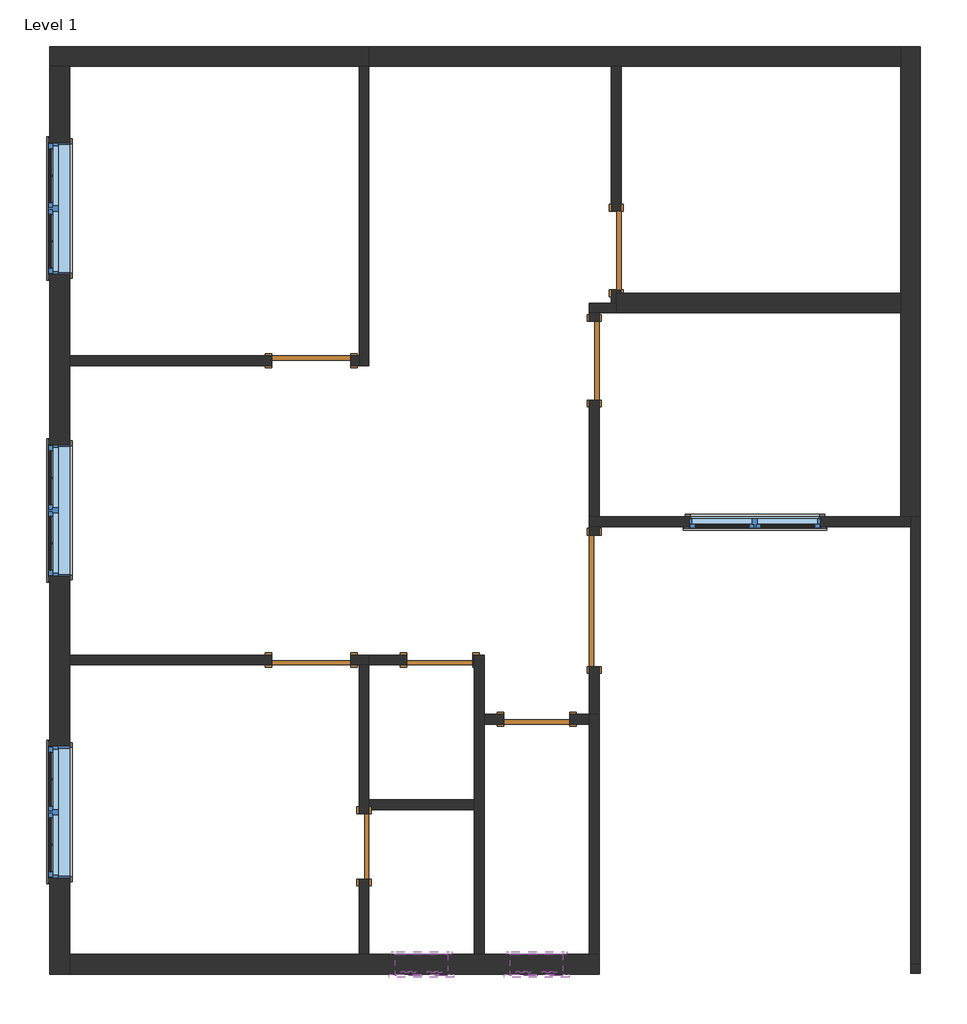
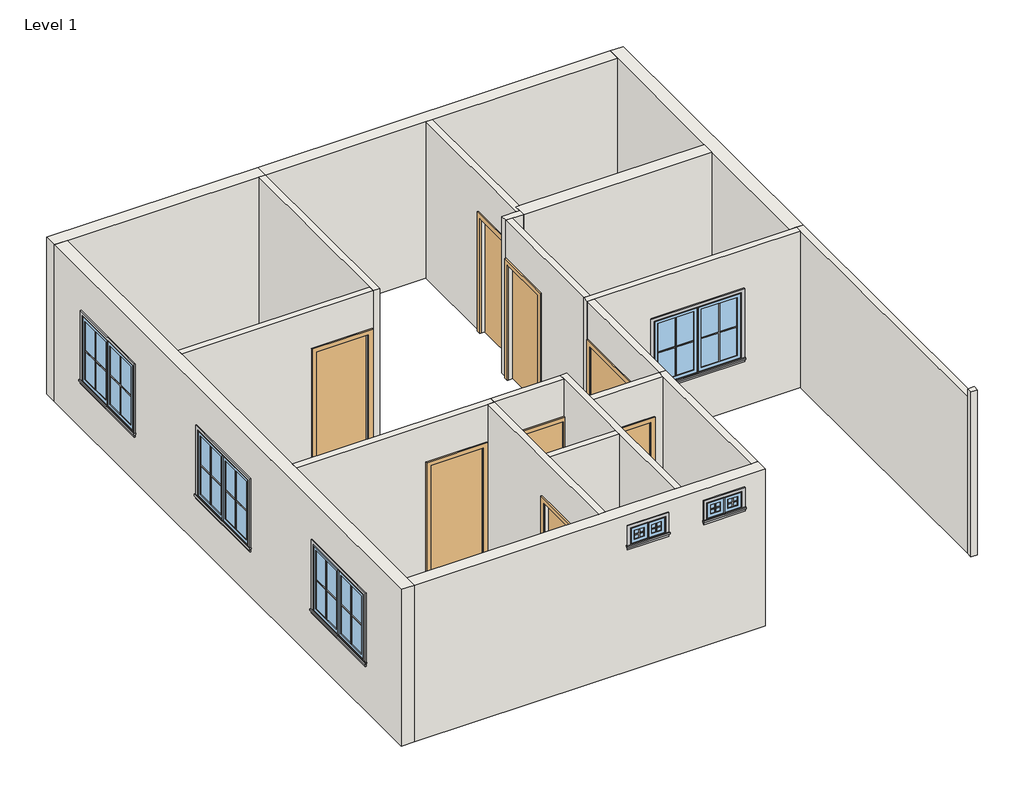
# One storey: 24 proxies, 22 walls, 8 doors, 6 windows.
"""IFC4 building model written with IfcOpenShell, lengths in millimetres."""

from ifc_helpers import new_model, si_unit, frame, origin, place, context, project, spatial, polyline, outline, extrude, faceted_brep, transform, mapped, element, save
from components import muntin_pattern_2x2_muntin_pattern_2x2_0a3992d1, muntin_pattern_2x2_muntin_pattern_2x2_f598e128, muntin_pattern_2x2_muntin_pattern_2x2_4939cdd6, muntin_pattern_2x2_muntin_pattern_2x2_7edc5815, trim_window_exterior_flat_with_sill_7631c5ba, trim_window_exterior_flat_with_sill_281d40e2, trim_window_interior_flat_picture_frame_0f2e31f9, trim_window_interior_flat_picture_frame_d1e4ee8f, door_214872d5, door_78caadf7, door_305aa2a5, door_e5f9f3c4, door_ea54c7da, window_375d1de9, window_9418cf83, window_178678fa

model = new_model("IFC4")

# Units and contexts
model_context = context("Model", 3, world=origin())
ifc_project = project(units=[si_unit("LENGTHUNIT", "METRE", prefix="MILLI")], contexts=[model_context])

# Site, building, storey
site = spatial("IfcSite", under=ifc_project)
building = spatial("IfcBuilding", under=site)
storey = spatial("IfcBuildingStorey", under=building, Name="Level 1", Elevation=609.6)

# Proxies
placement = place(None, origin())
muntin_pattern_2x2_muntin_pattern_2x2_shape = muntin_pattern_2x2_muntin_pattern_2x2_0a3992d1(model_context)
element("IfcBuildingElementProxy", 1, Name="Muntin Pattern_2x2 : Muntin Pattern_2x2", ObjectType="Muntin Pattern_2x2 : Muntin Pattern_2x2", at=placement, inside=storey, context=model_context, shape_type="MappedRepresentation", body=[
    mapped(muntin_pattern_2x2_muntin_pattern_2x2_shape, transform((-1063.8054063, 5260.5138401, 1593.85), x_axis=(-1.0, 0.0, 0.0), y_axis=(0.0, -1.0, 0.0), z_axis=(0.0, 0.0, 1.0))),
])
element("IfcBuildingElementProxy", 2, Name="Muntin Pattern_2x2 : Muntin Pattern_2x2", ObjectType="Muntin Pattern_2x2 : Muntin Pattern_2x2", at=placement, inside=storey, context=model_context, shape_type="MappedRepresentation", body=[
    mapped(muntin_pattern_2x2_muntin_pattern_2x2_shape, transform((-9599.7929063, 1566.4013401, 1593.85), x_axis=(0.0, 1.0, 0.0), y_axis=(-1.0, 0.0, 0.0), z_axis=(0.0, 0.0, 1.0))),
])
element("IfcBuildingElementProxy", 3, Name="Muntin Pattern_2x2 : Muntin Pattern_2x2", ObjectType="Muntin Pattern_2x2 : Muntin Pattern_2x2", at=placement, inside=storey, context=model_context, shape_type="MappedRepresentation", body=[
    mapped(muntin_pattern_2x2_muntin_pattern_2x2_shape, transform((-9599.7929063, 5062.0763401, 1593.85), x_axis=(0.0, 1.0, 0.0), y_axis=(-1.0, 0.0, 0.0), z_axis=(0.0, 0.0, 1.0))),
])
element("IfcBuildingElementProxy", 4, Name="Muntin Pattern_2x2 : Muntin Pattern_2x2", ObjectType="Muntin Pattern_2x2 : Muntin Pattern_2x2", at=placement, inside=storey, context=model_context, shape_type="MappedRepresentation", body=[
    mapped(muntin_pattern_2x2_muntin_pattern_2x2_shape, transform((-9599.7929063, 8557.7513401, 1593.85), x_axis=(0.0, 1.0, 0.0), y_axis=(-1.0, 0.0, 0.0), z_axis=(0.0, 0.0, 1.0))),
])
muntin_pattern_2x2_muntin_pattern_2x2_2_shape = muntin_pattern_2x2_muntin_pattern_2x2_f598e128(model_context)
element("IfcBuildingElementProxy", 5, Name="Muntin Pattern_2x2 : Muntin Pattern_2x2", ObjectType="Muntin Pattern_2x2 : Muntin Pattern_2x2", at=placement, inside=storey, context=model_context, shape_type="MappedRepresentation", body=[
    mapped(muntin_pattern_2x2_muntin_pattern_2x2_2_shape, transform((-1822.6304063, 5260.5138401, 1593.85), x_axis=(1.0, 0.0, 0.0), y_axis=(0.0, 1.0, 0.0), z_axis=(0.0, 0.0, 1.0))),
])
element("IfcBuildingElementProxy", 6, Name="Muntin Pattern_2x2 : Muntin Pattern_2x2", ObjectType="Muntin Pattern_2x2 : Muntin Pattern_2x2", at=placement, inside=storey, context=model_context, shape_type="MappedRepresentation", body=[
    mapped(muntin_pattern_2x2_muntin_pattern_2x2_2_shape, transform((-9599.7929063, 2325.2263401, 1593.85), x_axis=(0.0, -1.0, 0.0), y_axis=(1.0, 0.0, 0.0), z_axis=(0.0, 0.0, 1.0))),
])
element("IfcBuildingElementProxy", 7, Name="Muntin Pattern_2x2 : Muntin Pattern_2x2", ObjectType="Muntin Pattern_2x2 : Muntin Pattern_2x2", at=placement, inside=storey, context=model_context, shape_type="MappedRepresentation", body=[
    mapped(muntin_pattern_2x2_muntin_pattern_2x2_2_shape, transform((-9599.7929063, 5820.9013401, 1593.85), x_axis=(0.0, -1.0, 0.0), y_axis=(1.0, 0.0, 0.0), z_axis=(0.0, 0.0, 1.0))),
])
element("IfcBuildingElementProxy", 8, Name="Muntin Pattern_2x2 : Muntin Pattern_2x2", ObjectType="Muntin Pattern_2x2 : Muntin Pattern_2x2", at=placement, inside=storey, context=model_context, shape_type="MappedRepresentation", body=[
    mapped(muntin_pattern_2x2_muntin_pattern_2x2_2_shape, transform((-9599.7929063, 9316.5763401, 1593.85), x_axis=(0.0, -1.0, 0.0), y_axis=(1.0, 0.0, 0.0), z_axis=(0.0, 0.0, 1.0))),
])
muntin_pattern_2x2_muntin_pattern_2x2_3_shape = muntin_pattern_2x2_muntin_pattern_2x2_4939cdd6(model_context)
element("IfcBuildingElementProxy", 9, Name="Muntin Pattern_2x2 : Muntin Pattern_2x2", ObjectType="Muntin Pattern_2x2 : Muntin Pattern_2x2", at=placement, inside=storey, context=model_context, shape_type="MappedRepresentation", body=[
    mapped(muntin_pattern_2x2_muntin_pattern_2x2_3_shape, transform((-5153.2054063, 78.9138401, 3016.25), x_axis=(-1.0, 0.0, 0.0), y_axis=(0.0, -1.0, 0.0), z_axis=(0.0, 0.0, 1.0))),
])
element("IfcBuildingElementProxy", 10, Name="Muntin Pattern_2x2 : Muntin Pattern_2x2", ObjectType="Muntin Pattern_2x2 : Muntin Pattern_2x2", at=placement, inside=storey, context=model_context, shape_type="MappedRepresentation", body=[
    mapped(muntin_pattern_2x2_muntin_pattern_2x2_3_shape, transform((-3819.7054063, 78.9138401, 3016.25), x_axis=(-1.0, 0.0, 0.0), y_axis=(0.0, -1.0, 0.0), z_axis=(0.0, 0.0, 1.0))),
])
muntin_pattern_2x2_muntin_pattern_2x2_4_shape = muntin_pattern_2x2_muntin_pattern_2x2_7edc5815(model_context)
element("IfcBuildingElementProxy", 11, Name="Muntin Pattern_2x2 : Muntin Pattern_2x2", ObjectType="Muntin Pattern_2x2 : Muntin Pattern_2x2", at=placement, inside=storey, context=model_context, shape_type="MappedRepresentation", body=[
    mapped(muntin_pattern_2x2_muntin_pattern_2x2_4_shape, transform((-5454.8304063, 78.9138401, 3016.25), x_axis=(1.0, 0.0, 0.0), y_axis=(0.0, 1.0, 0.0), z_axis=(0.0, 0.0, 1.0))),
])
element("IfcBuildingElementProxy", 12, Name="Muntin Pattern_2x2 : Muntin Pattern_2x2", ObjectType="Muntin Pattern_2x2 : Muntin Pattern_2x2", at=placement, inside=storey, context=model_context, shape_type="MappedRepresentation", body=[
    mapped(muntin_pattern_2x2_muntin_pattern_2x2_4_shape, transform((-4121.3304063, 78.9138401, 3016.25), x_axis=(1.0, 0.0, 0.0), y_axis=(0.0, 1.0, 0.0), z_axis=(0.0, 0.0, 1.0))),
])
trim_window_exterior_flat_with_sill_shape = trim_window_exterior_flat_with_sill_7631c5ba(model_context)
element("IfcBuildingElementProxy", 13, Name="Trim-Window-Exterior-Flat : with Sill", ObjectType="Trim-Window-Exterior-Flat : with Sill", at=placement, inside=storey, context=model_context, shape_type="MappedRepresentation", body=[
    mapped(trim_window_exterior_flat_with_sill_shape, transform((-1443.2179063, 5250.9888401, 2743.2), x_axis=(1.0, 0.0, 0.0), y_axis=(0.0, 0.0, 1.0), z_axis=(0.0, -1.0, 0.0))),
])
element("IfcBuildingElementProxy", 14, Name="Trim-Window-Exterior-Flat : with Sill", ObjectType="Trim-Window-Exterior-Flat : with Sill", at=placement, inside=storey, context=model_context, shape_type="MappedRepresentation", body=[
    mapped(trim_window_exterior_flat_with_sill_shape, transform((-9609.3179063, 1945.8138401, 2743.2), x_axis=(0.0, -1.0, 0.0), y_axis=(0.0, 0.0, 1.0), z_axis=(-1.0, 0.0, 0.0))),
])
element("IfcBuildingElementProxy", 15, Name="Trim-Window-Exterior-Flat : with Sill", ObjectType="Trim-Window-Exterior-Flat : with Sill", at=placement, inside=storey, context=model_context, shape_type="MappedRepresentation", body=[
    mapped(trim_window_exterior_flat_with_sill_shape, transform((-9609.3179063, 5441.4888401, 2743.2), x_axis=(0.0, -1.0, 0.0), y_axis=(0.0, 0.0, 1.0), z_axis=(-1.0, 0.0, 0.0))),
])
element("IfcBuildingElementProxy", 16, Name="Trim-Window-Exterior-Flat : with Sill", ObjectType="Trim-Window-Exterior-Flat : with Sill", at=placement, inside=storey, context=model_context, shape_type="MappedRepresentation", body=[
    mapped(trim_window_exterior_flat_with_sill_shape, transform((-9609.3179063, 8937.1638401, 2743.2), x_axis=(0.0, -1.0, 0.0), y_axis=(0.0, 0.0, 1.0), z_axis=(-1.0, 0.0, 0.0))),
])
trim_window_exterior_flat_with_sill_2_shape = trim_window_exterior_flat_with_sill_281d40e2(model_context)
element("IfcBuildingElementProxy", 17, Name="Trim-Window-Exterior-Flat : with Sill", ObjectType="Trim-Window-Exterior-Flat : with Sill", at=placement, inside=storey, context=model_context, shape_type="MappedRepresentation", body=[
    mapped(trim_window_exterior_flat_with_sill_2_shape, transform((-5304.0179063, 69.3888401, 3251.2), x_axis=(1.0, 0.0, 0.0), y_axis=(0.0, 0.0, 1.0), z_axis=(0.0, -1.0, 0.0))),
])
element("IfcBuildingElementProxy", 18, Name="Trim-Window-Exterior-Flat : with Sill", ObjectType="Trim-Window-Exterior-Flat : with Sill", at=placement, inside=storey, context=model_context, shape_type="MappedRepresentation", body=[
    mapped(trim_window_exterior_flat_with_sill_2_shape, transform((-3970.5179063, 69.3888401, 3251.2), x_axis=(1.0, 0.0, 0.0), y_axis=(0.0, 0.0, 1.0), z_axis=(0.0, -1.0, 0.0))),
])
trim_window_interior_flat_picture_frame_shape = trim_window_interior_flat_picture_frame_0f2e31f9(model_context)
element("IfcBuildingElementProxy", 19, Name="Trim-Window-Interior-Flat : Picture Frame", ObjectType="Trim-Window-Interior-Flat : Picture Frame", at=placement, inside=storey, context=model_context, shape_type="MappedRepresentation", body=[
    mapped(trim_window_interior_flat_picture_frame_shape, transform((-1443.2179063, 5365.2888401, 2743.2), x_axis=(-1.0, 0.0, 0.0), y_axis=(0.0, 0.0, 1.0), z_axis=(0.0, 1.0, 0.0))),
])
element("IfcBuildingElementProxy", 20, Name="Trim-Window-Interior-Flat : Picture Frame", ObjectType="Trim-Window-Interior-Flat : Picture Frame", at=placement, inside=storey, context=model_context, shape_type="MappedRepresentation", body=[
    mapped(trim_window_interior_flat_picture_frame_shape, transform((-9380.7179063, 1945.8138401, 2743.2), x_axis=(0.0, 1.0, 0.0), y_axis=(0.0, 0.0, 1.0), z_axis=(1.0, 0.0, 0.0))),
])
element("IfcBuildingElementProxy", 21, Name="Trim-Window-Interior-Flat : Picture Frame", ObjectType="Trim-Window-Interior-Flat : Picture Frame", at=placement, inside=storey, context=model_context, shape_type="MappedRepresentation", body=[
    mapped(trim_window_interior_flat_picture_frame_shape, transform((-9380.7179063, 5441.4888401, 2743.2), x_axis=(0.0, 1.0, 0.0), y_axis=(0.0, 0.0, 1.0), z_axis=(1.0, 0.0, 0.0))),
])
element("IfcBuildingElementProxy", 22, Name="Trim-Window-Interior-Flat : Picture Frame", ObjectType="Trim-Window-Interior-Flat : Picture Frame", at=placement, inside=storey, context=model_context, shape_type="MappedRepresentation", body=[
    mapped(trim_window_interior_flat_picture_frame_shape, transform((-9380.7179063, 8937.1638401, 2743.2), x_axis=(0.0, 1.0, 0.0), y_axis=(0.0, 0.0, 1.0), z_axis=(1.0, 0.0, 0.0))),
])
trim_window_interior_flat_picture_frame_2_shape = trim_window_interior_flat_picture_frame_d1e4ee8f(model_context)
element("IfcBuildingElementProxy", 23, Name="Trim-Window-Interior-Flat : Picture Frame", ObjectType="Trim-Window-Interior-Flat : Picture Frame", at=placement, inside=storey, context=model_context, shape_type="MappedRepresentation", body=[
    mapped(trim_window_interior_flat_picture_frame_2_shape, transform((-5304.0179063, 297.9888401, 3251.2), x_axis=(-1.0, 0.0, 0.0), y_axis=(0.0, 0.0, 1.0), z_axis=(0.0, 1.0, 0.0))),
])
element("IfcBuildingElementProxy", 24, Name="Trim-Window-Interior-Flat : Picture Frame", ObjectType="Trim-Window-Interior-Flat : Picture Frame", at=placement, inside=storey, context=model_context, shape_type="MappedRepresentation", body=[
    mapped(trim_window_interior_flat_picture_frame_2_shape, transform((-3970.5179063, 297.9888401, 3251.2), x_axis=(-1.0, 0.0, 0.0), y_axis=(0.0, 0.0, 1.0), z_axis=(0.0, 1.0, 0.0))),
])

# Doors
door_shape = door_214872d5(model_context)
element("IfcDoor", 25, ObjectType="Single-Flush : 30\" x 84\"", at=placement, inside=storey, context=model_context, shape_type="MappedRepresentation", body=[
    mapped(door_shape, transform((-3970.5179063, 3022.1388401, 609.6), x_axis=(-1.0, 0.0, 0.0), y_axis=(0.0, -1.0, 0.0), z_axis=(0.0, 0.0, 1.0))),
])
door_2_shape = door_78caadf7(model_context)
element("IfcDoor", 26, ObjectType="Single-Flush : 30\" x 84\"", at=placement, inside=storey, context=model_context, shape_type="MappedRepresentation", body=[
    mapped(door_2_shape, transform((-5094.4679063, 3707.9388401, 609.6), x_axis=(1.0, 0.0, 0.0), y_axis=(0.0, 1.0, 0.0), z_axis=(0.0, 0.0, 1.0))),
])
element("IfcDoor", 27, ObjectType="Single-Flush : 30\" x 84\"", at=placement, inside=storey, context=model_context, shape_type="MappedRepresentation", body=[
    mapped(door_2_shape, transform((-5970.7679063, 1548.9388401, 609.6), x_axis=(0.0, 1.0, 0.0), y_axis=(-1.0, 0.0, 0.0), z_axis=(0.0, 0.0, 1.0))),
])
door_3_shape = door_305aa2a5(model_context)
element("IfcDoor", 28, ObjectType="Single-Flush : 36\" x 84\"", at=placement, inside=storey, context=model_context, shape_type="MappedRepresentation", body=[
    mapped(door_3_shape, transform((-6580.3679063, 3707.9388401, 609.6), x_axis=(1.0, 0.0, 0.0), y_axis=(0.0, 1.0, 0.0), z_axis=(0.0, 0.0, 1.0))),
])
element("IfcDoor", 29, ObjectType="Single-Flush : 36\" x 84\"", at=placement, inside=storey, context=model_context, shape_type="MappedRepresentation", body=[
    mapped(door_3_shape, transform((-3303.7679063, 7175.0388401, 609.6), x_axis=(0.0, 1.0, 0.0), y_axis=(-1.0, 0.0, 0.0), z_axis=(0.0, 0.0, 1.0))),
])
door_4_shape = door_e5f9f3c4(model_context)
element("IfcDoor", 30, ObjectType="Single-Flush : 36\" x 84\"", at=placement, inside=storey, context=model_context, shape_type="MappedRepresentation", body=[
    mapped(door_4_shape, transform((-3049.7679063, 8451.3888401, 609.6), x_axis=(0.0, -1.0, 0.0), y_axis=(1.0, 0.0, 0.0), z_axis=(0.0, 0.0, 1.0))),
])
element("IfcDoor", 31, ObjectType="Single-Flush : 36\" x 84\"", at=placement, inside=storey, context=model_context, shape_type="MappedRepresentation", body=[
    mapped(door_4_shape, transform((-6580.3679063, 7175.0388401, 609.6), x_axis=(1.0, 0.0, 0.0), y_axis=(0.0, 1.0, 0.0), z_axis=(0.0, 0.0, 1.0))),
])
door_5_shape = door_ea54c7da(model_context)
element("IfcDoor", 32, ObjectType="Single-Flush : 60\"x84\"", at=placement, inside=storey, context=model_context, shape_type="MappedRepresentation", body=[
    mapped(door_5_shape, transform((-3303.7679063, 4393.7388401, 609.6), x_axis=(0.0, 1.0, 0.0), y_axis=(-1.0, 0.0, 0.0), z_axis=(0.0, 0.0, 1.0))),
])

# Walls
element("IfcWall", 33, ObjectType="wall 4.5\"", at=placement, inside=storey, context=model_context, shape_type="Brep", body=[
    faceted_brep([(-6027.9179063, 10584.9888401, 609.6), (-6027.9179063, 7232.1888401, 609.6), (-6027.9179063, 7117.8888401, 609.6), (-6027.9179063, 7117.8888401, 3505.2), (-6027.9179063, 7232.1888401, 3505.2), (-6027.9179063, 10584.9888401, 3505.2), (-5913.6179063, 10584.9888401, 609.6), (-5913.6179063, 10584.9888401, 3505.2), (-5913.6179063, 7117.8888401, 3505.2), (-5913.6179063, 7117.8888401, 609.6)], [[[0, 1, 2, 3, 4, 5]], [[6, 7, 8, 9]], [[2, 1, 0, 6, 9]], [[0, 5, 7, 6]], [[3, 2, 9, 8]], [[5, 4, 3, 8, 7]]]),
])
element("IfcWall", 34, ObjectType="wall 4.5\"", at=placement, inside=storey, context=model_context, shape_type="SweptSolid", body=[
    extrude(outline(polyline([(2743.2, -6123.1679063), (609.6, -6123.1679063), (609.6, -6027.9179063), (3505.2, -6027.9179063), (3505.2, -9380.7179063), (609.6, -9380.7179063), (609.6, -7037.5679063), (2743.2, -7037.5679063), (2743.2, -6123.1679063)])), frame((0.0, 7117.8888401, 0.0), z_axis=(0.0, 1.0, 0.0), x_axis=(0.0, 0.0, 1.0)), (0.0, 0.0, 1.0), 114.3),
])
element("IfcWall", 35, ObjectType="wall 4.5\"", at=placement, inside=storey, context=model_context, shape_type="Brep", body=[
    faceted_brep([(-6123.1679063, 3650.7888401, 2743.2), (-6123.1679063, 3650.7888401, 609.6), (-6027.9179063, 3650.7888401, 609.6), (-5913.6179063, 3650.7888401, 609.6), (-5913.6179063, 3650.7888401, 3505.2), (-6027.9179063, 3650.7888401, 3505.2), (-9380.7179063, 3650.7888401, 3505.2), (-9380.7179063, 3650.7888401, 609.6), (-7037.5679063, 3650.7888401, 609.6), (-7037.5679063, 3650.7888401, 2743.2), (-5913.6179063, 3765.0888401, 609.6), (-6123.1679063, 3765.0888401, 609.6), (-6123.1679063, 3765.0888401, 2743.2), (-7037.5679063, 3765.0888401, 2743.2), (-7037.5679063, 3765.0888401, 609.6), (-9380.7179063, 3765.0888401, 609.6), (-9380.7179063, 3765.0888401, 3505.2), (-5913.6179063, 3765.0888401, 3505.2)], [[[0, 1, 2, 3, 4, 5, 6, 7, 8, 9]], [[10, 11, 12, 13, 14, 15, 16, 17]], [[8, 7, 15, 14]], [[3, 2, 1, 11, 10]], [[7, 6, 16, 15]], [[4, 3, 10, 17]], [[12, 11, 1, 0]], [[13, 12, 0, 9]], [[14, 13, 9, 8]], [[6, 5, 4, 17, 16]]]),
])
element("IfcWall", 36, ObjectType="wall 4.5\"", at=placement, inside=storey, context=model_context, shape_type="Brep", body=[
    faceted_brep([(-5913.6179063, 1929.9388401, 2743.2), (-5913.6179063, 1929.9388401, 609.6), (-5913.6179063, 1974.3888401, 609.6), (-5913.6179063, 2088.6888401, 609.6), (-5913.6179063, 3650.7888401, 609.6), (-5913.6179063, 3650.7888401, 3505.2), (-5913.6179063, 2088.6888401, 3505.2), (-5913.6179063, 1974.3888401, 3505.2), (-5913.6179063, 297.9888401, 3505.2), (-5913.6179063, 297.9888401, 609.6), (-5913.6179063, 1167.9388401, 609.6), (-5913.6179063, 1167.9388401, 2743.2), (-6027.9179063, 3650.7888401, 609.6), (-6027.9179063, 1929.9388401, 609.6), (-6027.9179063, 1929.9388401, 2743.2), (-6027.9179063, 1167.9388401, 2743.2), (-6027.9179063, 1167.9388401, 609.6), (-6027.9179063, 297.9888401, 609.6), (-6027.9179063, 297.9888401, 3505.2), (-6027.9179063, 3650.7888401, 3505.2)], [[[0, 1, 2, 3, 4, 5, 6, 7, 8, 9, 10, 11]], [[12, 13, 14, 15, 16, 17, 18, 19]], [[10, 9, 17, 16]], [[4, 3, 2, 1, 13, 12]], [[5, 4, 12, 19]], [[9, 8, 18, 17]], [[14, 13, 1, 0]], [[15, 14, 0, 11]], [[16, 15, 11, 10]], [[8, 7, 6, 5, 19, 18]]]),
])
element("IfcWall", 37, ObjectType="wall 4.5\"", at=placement, inside=storey, context=model_context, shape_type="Brep", body=[
    faceted_brep([(-4580.1179063, 297.9888401, 609.6), (-4580.1179063, 2964.9888401, 609.6), (-4580.1179063, 3079.2888401, 609.6), (-4580.1179063, 3765.0888401, 609.6), (-4580.1179063, 3765.0888401, 3505.2), (-4580.1179063, 3079.2888401, 3505.2), (-4580.1179063, 2964.9888401, 3505.2), (-4580.1179063, 297.9888401, 3505.2), (-4694.4179063, 297.9888401, 609.6), (-4694.4179063, 297.9888401, 3505.2), (-4694.4179063, 1974.3888401, 3505.2), (-4694.4179063, 2088.6888401, 3505.2), (-4694.4179063, 3650.7888401, 3505.2), (-4694.4179063, 3765.0888401, 3505.2), (-4694.4179063, 3765.0888401, 609.6), (-4694.4179063, 3650.7888401, 609.6), (-4694.4179063, 2088.6888401, 609.6), (-4694.4179063, 1974.3888401, 609.6)], [[[0, 1, 2, 3, 4, 5, 6, 7]], [[8, 9, 10, 11, 12, 13, 14, 15, 16, 17]], [[3, 2, 1, 0, 8, 17, 16, 15, 14]], [[0, 7, 9, 8]], [[4, 3, 14, 13]], [[7, 6, 5, 4, 13, 12, 11, 10, 9]]]),
])
element("IfcWall", 38, ObjectType="wall 4.5\"", at=placement, inside=storey, context=model_context, shape_type="SweptSolid", body=[
    extrude(outline(polyline([(-5913.6179063, 2088.6888401), (-4694.4179063, 2088.6888401), (-4694.4179063, 1974.3888401), (-5913.6179063, 1974.3888401), (-5913.6179063, 2088.6888401)])), frame((0.0, 0.0, 609.6), z_axis=(0.0, 0.0, 1.0), x_axis=(1.0, 0.0, 0.0)), (0.0, 0.0, 1.0), 2895.6),
])
element("IfcWall", 39, ObjectType="wall 4.5\"", at=placement, inside=storey, context=model_context, shape_type="SweptSolid", body=[
    extrude(outline(polyline([(2743.2, -4713.4679063), (609.6, -4713.4679063), (609.6, -4694.4179063), (3505.2, -4694.4179063), (3505.2, -5913.6179063), (609.6, -5913.6179063), (609.6, -5475.4679063), (2743.2, -5475.4679063), (2743.2, -4713.4679063)])), frame((0.0, 3650.7888401, 0.0), z_axis=(0.0, 1.0, 0.0), x_axis=(0.0, 0.0, 1.0)), (0.0, 0.0, 1.0), 114.3),
])
element("IfcWall", 40, ObjectType="wall 4.5\"", at=placement, inside=storey, context=model_context, shape_type="Brep", body=[
    faceted_brep([(-3246.6179063, 297.9888401, 609.6), (-3246.6179063, 3079.2888401, 609.6), (-3246.6179063, 3079.2888401, 3505.2), (-3246.6179063, 297.9888401, 3505.2), (-3360.9179063, 297.9888401, 609.6), (-3360.9179063, 297.9888401, 3505.2), (-3360.9179063, 2964.9888401, 3505.2), (-3360.9179063, 3079.2888401, 3505.2), (-3360.9179063, 3079.2888401, 609.6), (-3360.9179063, 2964.9888401, 609.6)], [[[0, 1, 2, 3]], [[4, 5, 6, 7, 8, 9]], [[1, 0, 4, 9, 8]], [[2, 1, 8, 7]], [[0, 3, 5, 4]], [[3, 2, 7, 6, 5]]]),
])
element("IfcWall", 41, ObjectType="wall 4.5\"", at=placement, inside=storey, context=model_context, shape_type="SweptSolid", body=[
    extrude(outline(polyline([(609.6, -4580.1179063), (609.6, -4351.5179063), (2743.2, -4351.5179063), (2743.2, -3589.5179063), (609.6, -3589.5179063), (609.6, -3360.9179063), (3505.2, -3360.9179063), (3505.2, -4580.1179063), (609.6, -4580.1179063)])), frame((0.0, 2964.9888401, 0.0), z_axis=(0.0, 1.0, 0.0), x_axis=(0.0, 0.0, 1.0)), (0.0, 0.0, 1.0), 114.3),
])
element("IfcWall", 42, ObjectType="wall 4.5\"", at=placement, inside=storey, context=model_context, shape_type="Brep", body=[
    faceted_brep([(474.4820937, 183.6888401, 609.6), (474.4820937, 5365.2888401, 609.6), (474.4820937, 5365.2888401, 3505.2), (474.4820937, 183.6888401, 3505.2), (360.1820937, 183.6888401, 609.6), (360.1820937, 183.6888401, 3505.2), (360.1820937, 5250.9888401, 3505.2), (360.1820937, 5365.2888401, 3505.2), (360.1820937, 5365.2888401, 609.6), (360.1820937, 5250.9888401, 609.6)], [[[0, 1, 2, 3]], [[4, 5, 6, 7, 8, 9]], [[1, 0, 4, 9, 8]], [[0, 3, 5, 4]], [[2, 1, 8, 7]], [[3, 2, 7, 6, 5]]]),
])
element("IfcWall", 43, ObjectType="wall 4.5\"", at=placement, inside=storey, context=model_context, shape_type="Brep", body=[
    faceted_brep([(360.1820937, 5365.2888401, 609.6), (245.8820937, 5365.2888401, 609.6), (-3246.6179063, 5365.2888401, 609.6), (-3360.9179063, 5365.2888401, 609.6), (-3360.9179063, 5365.2888401, 3505.2), (-3246.6179063, 5365.2888401, 3505.2), (245.8820937, 5365.2888401, 3505.2), (360.1820937, 5365.2888401, 3505.2), (-2205.2179063, 5365.2888401, 2743.2), (-2205.2179063, 5365.2888401, 1524.0), (-681.2179063, 5365.2888401, 1524.0), (-681.2179063, 5365.2888401, 2743.2), (360.1820937, 5250.9888401, 609.6), (360.1820937, 5250.9888401, 3505.2), (-3246.6179063, 5250.9888401, 3505.2), (-3360.9179063, 5250.9888401, 3505.2), (-3360.9179063, 5250.9888401, 609.6), (-3246.6179063, 5250.9888401, 609.6), (-2205.2179063, 5250.9888401, 2743.2), (-681.2179063, 5250.9888401, 2743.2), (-681.2179063, 5250.9888401, 1524.0), (-2205.2179063, 5250.9888401, 1524.0)], [[[0, 1, 2, 3, 4, 5, 6, 7], [8, 9, 10, 11]], [[12, 13, 14, 15, 16, 17], [18, 19, 20, 21]], [[3, 2, 1, 0, 12, 17, 16]], [[0, 7, 13, 12]], [[4, 3, 16, 15]], [[7, 6, 5, 4, 15, 14, 13]], [[9, 8, 18, 21]], [[10, 9, 21, 20]], [[11, 10, 20, 19]], [[8, 11, 19, 18]]]),
])
element("IfcWall", 44, ObjectType="wall 4.5\"", at=placement, inside=storey, context=model_context, shape_type="SweptSolid", body=[
    extrude(outline(polyline([(5250.9888401, 609.6), (5155.7388401, 609.6), (5155.7388401, 2743.2), (3631.7388401, 2743.2), (3631.7388401, 609.6), (3079.2888401, 609.6), (3079.2888401, 3505.2), (5250.9888401, 3505.2), (5250.9888401, 609.6)])), frame((-3360.9179063, 0.0, 0.0), z_axis=(1.0, 0.0, 0.0), x_axis=(0.0, 1.0, 0.0)), (0.0, 0.0, 1.0), 114.3),
])
element("IfcWall", 45, ObjectType="wall 4.5\"", at=placement, inside=storey, context=model_context, shape_type="Brep", body=[
    faceted_brep([(-2992.6179063, 7956.0888401, 609.6), (-2992.6179063, 7994.1888401, 609.6), (-2992.6179063, 7994.1888401, 2743.2), (-2992.6179063, 8908.5888401, 2743.2), (-2992.6179063, 8908.5888401, 609.6), (-2992.6179063, 10584.9888401, 609.6), (-2992.6179063, 10584.9888401, 3505.2), (-2992.6179063, 7956.0888401, 3505.2), (-3106.9179063, 7994.1888401, 2743.2), (-3106.9179063, 7994.1888401, 609.6), (-3106.9179063, 7841.7888401, 609.6), (-3106.9179063, 7841.7888401, 3505.2), (-3106.9179063, 10584.9888401, 3505.2), (-3106.9179063, 10584.9888401, 609.6), (-3106.9179063, 8908.5888401, 609.6), (-3106.9179063, 8908.5888401, 2743.2), (-3049.7679063, 7956.0888401, 609.6), (-3049.7679063, 7841.7888401, 609.6), (-3049.7679063, 7956.0888401, 3505.2), (-3049.7679063, 7841.7888401, 3505.2)], [[[0, 1, 2, 3, 4, 5, 6, 7]], [[8, 9, 10, 11, 12, 13, 14, 15]], [[14, 13, 5, 4]], [[10, 9, 1, 0, 16, 17]], [[6, 5, 13, 12]], [[2, 1, 9, 8]], [[3, 2, 8, 15]], [[4, 3, 15, 14]], [[0, 7, 18, 16]], [[18, 19, 17, 16]], [[19, 11, 10, 17]], [[7, 6, 12, 11, 19, 18]]]),
])
element("IfcWall", 46, ObjectType="wall 4.5\"", at=placement, inside=storey, context=model_context, shape_type="SweptSolid", body=[
    extrude(outline(polyline([(7727.4888401, 609.6), (7632.2388401, 609.6), (7632.2388401, 2743.2), (6717.8388401, 2743.2), (6717.8388401, 609.6), (5365.2888401, 609.6), (5365.2888401, 3505.2), (7727.4888401, 3505.2), (7727.4888401, 609.6)])), frame((-3360.9179063, 0.0, 0.0), z_axis=(1.0, 0.0, 0.0), x_axis=(0.0, 1.0, 0.0)), (0.0, 0.0, 1.0), 114.3),
])
element("IfcWall", 47, ObjectType="wall 4.5\"", at=placement, inside=storey, context=model_context, shape_type="Brep", body=[
    faceted_brep([(-3049.7679063, 7841.7888401, 609.6), (-3106.9179063, 7841.7888401, 609.6), (-3360.9179063, 7841.7888401, 609.6), (-3360.9179063, 7841.7888401, 3505.2), (-3106.9179063, 7841.7888401, 3505.2), (-3049.7679063, 7841.7888401, 3505.2), (-3049.7679063, 7727.4888401, 609.6), (-3049.7679063, 7727.4888401, 3505.2), (-3246.6179063, 7727.4888401, 3505.2), (-3360.9179063, 7727.4888401, 3505.2), (-3360.9179063, 7727.4888401, 609.6), (-3246.6179063, 7727.4888401, 609.6)], [[[0, 1, 2, 3, 4, 5]], [[6, 7, 8, 9, 10, 11]], [[2, 1, 0, 6, 11, 10]], [[0, 5, 7, 6]], [[3, 2, 10, 9]], [[5, 4, 3, 9, 8, 7]]]),
])
element("IfcWall", 48, ObjectType="wall 4.5\"", at=placement, inside=storey, context=model_context, shape_type="Brep", body=[
    faceted_brep([(360.1820937, 183.6888401, 609.6), (360.1820937, 82.0888401, 609.6), (360.1820937, 82.0888401, 3657.6), (360.1820937, 183.6888401, 3657.6), (360.1820937, 183.6888401, 3505.2), (474.4820937, 183.6888401, 609.6), (474.4820937, 183.6888401, 3505.2), (474.4820937, 183.6888401, 3657.6), (474.4820937, 82.0888401, 3657.6), (474.4820937, 82.0888401, 609.6)], [[[0, 1, 2, 3, 4]], [[5, 6, 7, 8, 9]], [[1, 0, 5, 9]], [[2, 1, 9, 8]], [[3, 2, 8, 7]], [[0, 4, 3, 7, 6, 5]]]),
])
element("IfcWall", 49, ObjectType="wall 9\"", at=placement, inside=storey, context=model_context, shape_type="Brep", body=[
    faceted_brep([(-9609.3179063, 10584.9888401, 609.6), (-9380.7179063, 10584.9888401, 609.6), (-6027.9179063, 10584.9888401, 609.6), (-5913.6179063, 10584.9888401, 609.6), (-5913.6179063, 10584.9888401, 3505.2), (-6027.9179063, 10584.9888401, 3505.2), (-9380.7179063, 10584.9888401, 3505.2), (-9609.3179063, 10584.9888401, 3505.2), (-9609.3179063, 10813.5888401, 609.6), (-9609.3179063, 10813.5888401, 3505.2), (-5913.6179063, 10813.5888401, 3505.2), (-5913.6179063, 10813.5888401, 609.6)], [[[0, 1, 2, 3, 4, 5, 6, 7]], [[8, 9, 10, 11]], [[3, 2, 1, 0, 8, 11]], [[0, 7, 9, 8]], [[4, 3, 11, 10]], [[7, 6, 5, 4, 10, 9]]]),
])
element("IfcWall", 50, ObjectType="wall 9\"", at=placement, inside=storey, context=model_context, shape_type="Brep", body=[
    faceted_brep([(-9609.3179063, 10584.9888401, 609.6), (-9609.3179063, 69.3888401, 609.6), (-9609.3179063, 69.3888401, 3505.2), (-9609.3179063, 10584.9888401, 3505.2), (-9609.3179063, 2707.8138401, 2743.2), (-9609.3179063, 1183.8138401, 2743.2), (-9609.3179063, 1183.8138401, 1524.0), (-9609.3179063, 2707.8138401, 1524.0), (-9609.3179063, 6203.4888401, 2743.2), (-9609.3179063, 4679.4888401, 2743.2), (-9609.3179063, 4679.4888401, 1524.0), (-9609.3179063, 6203.4888401, 1524.0), (-9609.3179063, 9699.1638401, 2743.2), (-9609.3179063, 8175.1638401, 2743.2), (-9609.3179063, 8175.1638401, 1524.0), (-9609.3179063, 9699.1638401, 1524.0), (-9380.7179063, 10584.9888401, 609.6), (-9380.7179063, 10584.9888401, 3505.2), (-9380.7179063, 7232.1888401, 3505.2), (-9380.7179063, 7117.8888401, 3505.2), (-9380.7179063, 3765.0888401, 3505.2), (-9380.7179063, 3650.7888401, 3505.2), (-9380.7179063, 297.9888401, 3505.2), (-9380.7179063, 69.3888401, 3505.2), (-9380.7179063, 69.3888401, 609.6), (-9380.7179063, 297.9888401, 609.6), (-9380.7179063, 3650.7888401, 609.6), (-9380.7179063, 3765.0888401, 609.6), (-9380.7179063, 7117.8888401, 609.6), (-9380.7179063, 7232.1888401, 609.6), (-9380.7179063, 2707.8138401, 2743.2), (-9380.7179063, 2707.8138401, 1524.0), (-9380.7179063, 1183.8138401, 1524.0), (-9380.7179063, 1183.8138401, 2743.2), (-9380.7179063, 6203.4888401, 2743.2), (-9380.7179063, 6203.4888401, 1524.0), (-9380.7179063, 4679.4888401, 1524.0), (-9380.7179063, 4679.4888401, 2743.2), (-9380.7179063, 9699.1638401, 2743.2), (-9380.7179063, 9699.1638401, 1524.0), (-9380.7179063, 8175.1638401, 1524.0), (-9380.7179063, 8175.1638401, 2743.2)], [[[0, 1, 2, 3], [4, 5, 6, 7], [8, 9, 10, 11], [12, 13, 14, 15]], [[16, 17, 18, 19, 20, 21, 22, 23, 24, 25, 26, 27, 28, 29], [30, 31, 32, 33], [34, 35, 36, 37], [38, 39, 40, 41]], [[1, 0, 16, 29, 28, 27, 26, 25, 24]], [[0, 3, 17, 16]], [[2, 1, 24, 23]], [[3, 2, 23, 22, 21, 20, 19, 18, 17]], [[31, 30, 4, 7]], [[32, 31, 7, 6]], [[33, 32, 6, 5]], [[30, 33, 5, 4]], [[35, 34, 8, 11]], [[36, 35, 11, 10]], [[37, 36, 10, 9]], [[34, 37, 9, 8]], [[39, 38, 12, 15]], [[40, 39, 15, 14]], [[41, 40, 14, 13]], [[38, 41, 13, 12]]]),
])
element("IfcWall", 51, ObjectType="wall 9\"", at=placement, inside=storey, context=model_context, shape_type="Brep", body=[
    faceted_brep([(-9380.7179063, 69.3888401, 609.6), (-3246.6179063, 69.3888401, 609.6), (-3246.6179063, 69.3888401, 3505.2), (-9380.7179063, 69.3888401, 3505.2), (-5608.8179063, 69.3888401, 3251.2), (-4999.2179063, 69.3888401, 3251.2), (-4999.2179063, 69.3888401, 2946.4), (-5608.8179063, 69.3888401, 2946.4), (-4275.3179063, 69.3888401, 3251.2), (-3665.7179063, 69.3888401, 3251.2), (-3665.7179063, 69.3888401, 2946.4), (-4275.3179063, 69.3888401, 2946.4), (-9380.7179063, 297.9888401, 609.6), (-9380.7179063, 297.9888401, 3505.2), (-6027.9179063, 297.9888401, 3505.2), (-5913.6179063, 297.9888401, 3505.2), (-4694.4179063, 297.9888401, 3505.2), (-4580.1179063, 297.9888401, 3505.2), (-3360.9179063, 297.9888401, 3505.2), (-3246.6179063, 297.9888401, 3505.2), (-3246.6179063, 297.9888401, 609.6), (-3360.9179063, 297.9888401, 609.6), (-4580.1179063, 297.9888401, 609.6), (-4694.4179063, 297.9888401, 609.6), (-5913.6179063, 297.9888401, 609.6), (-6027.9179063, 297.9888401, 609.6), (-5608.8179063, 297.9888401, 3251.2), (-5608.8179063, 297.9888401, 2946.4), (-4999.2179063, 297.9888401, 2946.4), (-4999.2179063, 297.9888401, 3251.2), (-4275.3179063, 297.9888401, 3251.2), (-4275.3179063, 297.9888401, 2946.4), (-3665.7179063, 297.9888401, 2946.4), (-3665.7179063, 297.9888401, 3251.2)], [[[0, 1, 2, 3], [4, 5, 6, 7], [8, 9, 10, 11]], [[12, 13, 14, 15, 16, 17, 18, 19, 20, 21, 22, 23, 24, 25], [26, 27, 28, 29], [30, 31, 32, 33]], [[1, 0, 12, 25, 24, 23, 22, 21, 20]], [[0, 3, 13, 12]], [[2, 1, 20, 19]], [[3, 2, 19, 18, 17, 16, 15, 14, 13]], [[27, 26, 4, 7]], [[28, 27, 7, 6]], [[29, 28, 6, 5]], [[26, 29, 5, 4]], [[31, 30, 8, 11]], [[32, 31, 11, 10]], [[33, 32, 10, 9]], [[30, 33, 9, 8]]]),
])
element("IfcWall", 52, ObjectType="wall 9\"", at=placement, inside=storey, context=model_context, shape_type="Brep", body=[
    faceted_brep([(474.4820937, 5365.2888401, 609.6), (474.4820937, 10813.5888401, 609.6), (474.4820937, 10813.5888401, 3505.2), (474.4820937, 5365.2888401, 3505.2), (245.8820937, 5365.2888401, 609.6), (245.8820937, 5365.2888401, 3505.2), (245.8820937, 7727.4888401, 3505.2), (245.8820937, 7956.0888401, 3505.2), (245.8820937, 10584.9888401, 3505.2), (245.8820937, 10813.5888401, 3505.2), (245.8820937, 10813.5888401, 609.6), (245.8820937, 10584.9888401, 609.6), (245.8820937, 7956.0888401, 609.6), (245.8820937, 7727.4888401, 609.6), (360.1820937, 5365.2888401, 609.6), (360.1820937, 5365.2888401, 3505.2), (449.0820937, 10813.5888401, 3505.2)], [[[0, 1, 2, 3]], [[4, 5, 6, 7, 8, 9, 10, 11, 12, 13]], [[1, 0, 14, 4, 13, 12, 11, 10]], [[0, 3, 15, 5, 4, 14]], [[2, 1, 10, 9, 16]], [[3, 2, 16, 9, 8, 7, 6, 5, 15]]]),
])
element("IfcWall", 53, ObjectType="wall 9\"", at=placement, inside=storey, context=model_context, shape_type="Brep", body=[
    faceted_brep([(245.8820937, 7956.0888401, 609.6), (-2992.6179063, 7956.0888401, 609.6), (-3049.7679063, 7956.0888401, 609.6), (-3049.7679063, 7956.0888401, 3505.2), (-2992.6179063, 7956.0888401, 3505.2), (245.8820937, 7956.0888401, 3505.2), (245.8820937, 7727.4888401, 609.6), (245.8820937, 7727.4888401, 3505.2), (-3049.7679063, 7727.4888401, 3505.2), (-3049.7679063, 7727.4888401, 609.6), (-3049.7679063, 7841.7888401, 609.6), (-3049.7679063, 7841.7888401, 3505.2)], [[[0, 1, 2, 3, 4, 5]], [[6, 7, 8, 9]], [[2, 1, 0, 6, 9, 10]], [[3, 2, 10, 9, 8, 11]], [[0, 5, 7, 6]], [[5, 4, 3, 11, 8, 7]]]),
])
element("IfcWall", 54, ObjectType="wall 9\"", at=placement, inside=storey, context=model_context, shape_type="Brep", body=[
    faceted_brep([(245.8820937, 10813.5888401, 609.6), (-5913.6179063, 10813.5888401, 609.6), (-5913.6179063, 10813.5888401, 3505.2), (245.8820937, 10813.5888401, 3505.2), (245.8820937, 10584.9888401, 609.6), (245.8820937, 10584.9888401, 3505.2), (-2992.6179063, 10584.9888401, 3505.2), (-3106.9179063, 10584.9888401, 3505.2), (-5913.6179063, 10584.9888401, 3505.2), (-5913.6179063, 10584.9888401, 609.6), (-3106.9179063, 10584.9888401, 609.6), (-2992.6179063, 10584.9888401, 609.6)], [[[0, 1, 2, 3]], [[4, 5, 6, 7, 8, 9, 10, 11]], [[1, 0, 4, 11, 10, 9]], [[0, 3, 5, 4]], [[2, 1, 9, 8]], [[3, 2, 8, 7, 6, 5]]]),
])

# Windows
window_shape = window_375d1de9(model_context)
element("IfcWindow", 55, ObjectType="Window-Casement-Double : 24\"X1'", at=placement, inside=storey, context=model_context, shape_type="MappedRepresentation", body=[
    mapped(window_shape, transform((-5304.0179063, 183.6888401, 2032.0), x_axis=(-1.0, 0.0, 0.0), y_axis=(0.0, -1.0, 0.0), z_axis=(0.0, 0.0, 1.0))),
])
element("IfcWindow", 56, ObjectType="Window-Casement-Double : 24\"X1'", at=placement, inside=storey, context=model_context, shape_type="MappedRepresentation", body=[
    mapped(window_shape, transform((-3970.5179063, 183.6888401, 2032.0), x_axis=(-1.0, 0.0, 0.0), y_axis=(0.0, -1.0, 0.0), z_axis=(0.0, 0.0, 1.0))),
])
window_2_shape = window_9418cf83(model_context)
element("IfcWindow", 57, ObjectType="Window-Casement-Double : 60\"X48\"", at=placement, inside=storey, context=model_context, shape_type="MappedRepresentation", body=[
    mapped(window_2_shape, transform((-1443.2179063, 5308.1388401, 609.6), x_axis=(-1.0, 0.0, 0.0), y_axis=(0.0, -1.0, 0.0), z_axis=(0.0, 0.0, 1.0))),
])
window_3_shape = window_178678fa(model_context)
element("IfcWindow", 58, ObjectType="Window-Casement-Double : 60\"X48\"", at=placement, inside=storey, context=model_context, shape_type="MappedRepresentation", body=[
    mapped(window_3_shape, transform((-9495.0179063, 1945.8138401, 609.6), x_axis=(0.0, 1.0, 0.0), y_axis=(-1.0, 0.0, 0.0), z_axis=(0.0, 0.0, 1.0))),
])
element("IfcWindow", 59, ObjectType="Window-Casement-Double : 60\"X48\"", at=placement, inside=storey, context=model_context, shape_type="MappedRepresentation", body=[
    mapped(window_3_shape, transform((-9495.0179063, 5441.4888401, 609.6), x_axis=(0.0, 1.0, 0.0), y_axis=(-1.0, 0.0, 0.0), z_axis=(0.0, 0.0, 1.0))),
])
element("IfcWindow", 60, ObjectType="Window-Casement-Double : 60\"X48\"", at=placement, inside=storey, context=model_context, shape_type="MappedRepresentation", body=[
    mapped(window_3_shape, transform((-9495.0179063, 8937.1638401, 609.6), x_axis=(0.0, 1.0, 0.0), y_axis=(-1.0, 0.0, 0.0), z_axis=(0.0, 0.0, 1.0))),
])

save(model, "model.ifc")

# Revit data of these elements
# Type "Muntin Pattern_2x2 : Muntin Pattern_2x2"
#   Width [instance default] = 4' - 0"
#   Thickness = 0' - 0 1/2"
#   Height [instance default] = 4' - 0"
#   Distance = 0' - 0 3/4"
#   Interior Material [instance default] = none
#   Exterior Material [instance default] = none
#   Default Elevation = 0
# Type "Trim-Window-Exterior-Flat : with Sill"
#   Trim Width = 0' - 2 1/4"
#   Trim Thickness_Picture Frame = 0' - 1 1/4"
#   Trim Thickness_with Sill = 0' - 0 3/4"
#   Sill Thickness = 0' - 1 1/4"
#   Opening Width [instance default] = 2' - 0"
#   Opening Height [instance default] = 3' - 0"
#   Default Elevation = 4' - 0"
#   Sill = yes
#   Picture Frame = no
#   Trim Material [instance default] = none
# Type "Trim-Window-Interior-Flat : Picture Frame"
#   Trim Thickness_Picture Frame = 0' - 1 1/4"
#   Trim Width = 0' - 2 1/4"
#   Trim Thickness_with Sill = 0' - 0 3/4"
#   Sill Thickness = 0' - 1 1/4"
#   Opening Width [instance default] = 2' - 0"
#   Opening Height [instance default] = 3' - 0"
#   Default Elevation = 4' - 0"
#   Sill = no
#   Picture Frame = yes
#   Trim Material [instance default] = none
# Type "Single-Flush : 30\" x 84\""
#   Type Mark = "4"
#   Construction Type Id = "MDOOR"
#   Assembly Code = "C1020"
#   Analytic Construction = "Metal"
#   Thickness = 0' - 2"
#   Heat Transfer Coefficient (U) = 0.651978 BTU/(h·ft²·°F)
#   Height = 7' - 0"
#   Trim Projection Ext = 0' - 1"
#   Trim Projection Int = 0' - 1"
#   Trim Width = 0' - 3"
#   Width = 2' - 6"
#   Define Thermal Properties by = 1
#   Define Thermal Properties by = 1
#   Door Material = Door - Panel
#   Frame Material = Door - Frame
#   Visual Light Transmittance = 0
#   Solar Heat Gain Coefficient = 0
#   Function = (empty or 0)
#   Wall Closure = (empty or 0)
# Type "Single-Flush : 36\" x 84\""
#   Type Mark = "1"
#   Construction Type Id = "MDOOR"
#   Assembly Code = "C1020"
#   Analytic Construction = "Metal"
#   Thickness = 0' - 2"
#   Heat Transfer Coefficient (U) = 0.651978 BTU/(h·ft²·°F)
#   Height = 7' - 0"
#   Trim Projection Ext = 0' - 1"
#   Trim Projection Int = 0' - 1"
#   Trim Width = 0' - 3"
#   Width = 3' - 0"
#   Define Thermal Properties by = 1
#   Define Thermal Properties by = 1
#   Door Material = Door - Panel
#   Frame Material = Door - Frame
#   Visual Light Transmittance = 0
#   Solar Heat Gain Coefficient = 0
#   Function = (empty or 0)
#   Wall Closure = (empty or 0)
# Type "Single-Flush : 60\"x84\""
#   Type Mark = "8"
#   Construction Type Id = "MDOOR"
#   Assembly Code = "C1020"
#   Analytic Construction = "Metal"
#   Thickness = 0' - 2"
#   Heat Transfer Coefficient (U) = 0.651978 BTU/(h·ft²·°F)
#   Height = 7' - 0"
#   Trim Projection Ext = 0' - 1"
#   Trim Projection Int = 0' - 1"
#   Trim Width = 0' - 3"
#   Width = 5' - 0"
#   Define Thermal Properties by = 1
#   Door Material = Door - Panel
#   Frame Material = Door - Frame
#   Visual Light Transmittance = 0
#   Solar Heat Gain Coefficient = 0
#   Function = (empty or 0)
#   Wall Closure = (empty or 0)
# Type "wall 4.5\""
#   Assembly Code = "B2010"
#   Layers, outside or top first: 0' - 4 1/2" no material (function 1)
# Type "wall 9\""
#   Assembly Code = "B2010"
#   Layers, outside or top first: 0' - 9" no material (function 1)
# Type "Window-Casement-Double : 24\"X1'"
#   Type Mark = "V"
#   Fire Rating = "0.5h"
#   Assembly Code = "B2020100"
#   Analytic Construction = "Double glazing - domestic"
#   Frame Extension [instance default] = 0' - 0 1/4"
#   Window Inset [instance default] = 0' - 0"
#   Wall Thickness [instance default] = 0' - 6"
#   Interior Wall Closure [instance default] = 0' - 2 1/4"
#   Half Width = 1' - 0"
#   Visual Light Transmittance = 0.81
#   Thermal Resistance (R) = 1.8146 (h·ft²·°F)/BTU
#   Solar Heat Gain Coefficient = 0.76
#   Rough Width = 2' - 0 1/2"
#   Rough Height = 1' - 0 1/2"
#   Height = 1' - 0"
#   Heat Transfer Coefficient (U) = 0.5511 BTU/(h·ft²·°F)
#   Exterior Wall Closure [instance default] = 0' - 1 1/4"
#   Extension Jamb [instance default] = 0' - 2 1/4"
#   Default Sill Height = 3' - 0"
#   Width = 2' - 0"
#   Muntin Visibility = yes
#   Interior Trim Visibility [instance default] = yes
#   Exterior Trim Visibility [instance default] = yes
#   Extension Jamb Visibility [instance default] = yes
#   Interior Trim Material = Wood - Stained
#   Muntin Pattern = Muntin Pattern_2x2 : Muntin Pattern_2x2
#   Interior Trim = Trim-Window-Interior-Flat : Picture Frame
#   Interior Frame Material = Wood - Stained
#   Glass Panel Material = Glass
#   Exterior Trim Material = Clad - White
#   Exterior Trim = Trim-Window-Exterior-Flat : with Sill
#   Exterior Frame Material = Clad - White
#   Wall Closure = (empty or 0)
# Type "Window-Casement-Double : 60\"X48\""
#   Type Mark = "W"
#   Fire Rating = "0.5h"
#   Assembly Code = "B2020100"
#   Analytic Construction = "Double glazing - domestic"
#   Frame Extension [instance default] = 0' - 0 1/4"
#   Window Inset [instance default] = 0' - 0"
#   Wall Thickness [instance default] = 0' - 6"
#   Interior Wall Closure [instance default] = 0' - 2 1/4"
#   Half Width = 2' - 6"
#   Visual Light Transmittance = 0.81
#   Thermal Resistance (R) = 1.8146 (h·ft²·°F)/BTU
#   Solar Heat Gain Coefficient = 0.76
#   Rough Width = 5' - 0 1/2"
#   Rough Height = 4' - 0 1/2"
#   Height = 4' - 0"
#   Heat Transfer Coefficient (U) = 0.5511 BTU/(h·ft²·°F)
#   Exterior Wall Closure [instance default] = 0' - 1 1/4"
#   Extension Jamb [instance default] = 0' - 2 1/4"
#   Default Sill Height = 3' - 0"
#   Width = 5' - 0"
#   Muntin Visibility = yes
#   Interior Trim Visibility [instance default] = yes
#   Exterior Trim Visibility [instance default] = yes
#   Extension Jamb Visibility [instance default] = yes
#   Interior Trim Material = Wood - Stained
#   Muntin Pattern = Muntin Pattern_2x2 : Muntin Pattern_2x2
#   Interior Trim = Trim-Window-Interior-Flat : Picture Frame
#   Interior Frame Material = Wood - Stained
#   Glass Panel Material = Glass
#   Exterior Trim Material = Clad - White
#   Exterior Trim = Trim-Window-Exterior-Flat : with Sill
#   Exterior Frame Material = Clad - White
#   Wall Closure = (empty or 0)
# Elements 1, 2, 3, 4, 5, 6, 7, 8 (IfcBuildingElementProxy, "Muntin Pattern_2x2 : Muntin Pattern_2x2")
#   Width = 2' - 0 5/8"
#   Height = 3' - 6 1/2"
#   Interior Material = Wood - Stained
#   Exterior Material = Clad - White
#   Phase Created = New Construction
#   Materials on its faces: "Clad - White", "Wood - Stained"
# Elements 9, 10, 11, 12 (IfcBuildingElementProxy, "Muntin Pattern_2x2 : Muntin Pattern_2x2")
#   Width = 0' - 6 5/8"
#   Height = 0' - 6 1/2"
#   Interior Material = Wood - Stained
#   Exterior Material = Clad - White
#   Phase Created = New Construction
#   Materials on its faces: "Clad - White", "Wood - Stained"
# Elements 13, 14, 15, 16 (IfcBuildingElementProxy, "Trim-Window-Exterior-Flat : with Sill")
#   Opening Width = 5' - 0"
#   Opening Height = 4' - 0"
#   Trim Material = Clad - White
#   Phase Created = New Construction
#   Materials on its faces: "Clad - White"
# Elements 17, 18 (IfcBuildingElementProxy, "Trim-Window-Exterior-Flat : with Sill")
#   Opening Width = 2' - 0"
#   Opening Height = 1' - 0"
#   Trim Material = Clad - White
#   Phase Created = New Construction
#   Materials on its faces: "Clad - White"
# Elements 19, 20, 21, 22 (IfcBuildingElementProxy, "Trim-Window-Interior-Flat : Picture Frame")
#   Opening Width = 5' - 0"
#   Opening Height = 4' - 0"
#   Trim Material = Wood - Stained
#   Phase Created = New Construction
#   Materials on its faces: "Wood - Stained"
# Elements 23, 24 (IfcBuildingElementProxy, "Trim-Window-Interior-Flat : Picture Frame")
#   Opening Width = 2' - 0"
#   Opening Height = 1' - 0"
#   Trim Material = Wood - Stained
#   Phase Created = New Construction
#   Materials on its faces: "Wood - Stained"
# Elements 25, 26, 27 (IfcDoor, "Single-Flush : 30\" x 84\"")
#   Phase Created = New Construction
#   Materials on its faces: "Door - Frame", "Door - Panel"
# Elements 28, 29, 30, 31 (IfcDoor, "Single-Flush : 36\" x 84\"")
#   Phase Created = New Construction
#   Materials on its faces: "Door - Frame", "Door - Panel"
# Element 32 (IfcDoor, "Single-Flush : 60\"x84\"")
#   Phase Created = New Construction
#   Materials on its faces: "Door - Frame", "Door - Panel"
# Elements 33, 34, 35, 36, 37, 38, 39, 40, 41, 42, 43, 44, 45, 46, 47 (IfcWall, "wall 4.5\"")
#   Top Offset = 0' - 0"
#   Base Offset = 0' - 0"
#   wall height = 9' - 6"
#   Phase Created = New Construction
#   Base Constraint = Level 1
#   Top Constraint = SLAB
#   Materials on its faces: "Default Wall"
# Element 48 (IfcWall, "wall 4.5\"")
#   Top Offset = 0' - 0"
#   Base Offset = 0' - 0"
#   wall height = 10' - 0"
#   Phase Created = New Construction
#   Base Constraint = Level 1
#   Top Constraint = SLAB
#   Materials on its faces: "Default Wall"
# Elements 49, 50, 51, 52, 53, 54 (IfcWall, "wall 9\"")
#   Top Offset = 0' - 0"
#   Base Offset = 0' - 0"
#   wall height = 9' - 6"
#   Phase Created = New Construction
#   Base Constraint = Level 1
#   Top Constraint = SLAB
#   Materials on its faces: "Default Wall"
# Element 55 (IfcWindow, "Window-Casement-Double : 24\"X1'")
#   Mark = "7"
#   Window Inset = 0' - 0"
#   Interior Wall Closure = 0' - 2 1/4"
#   Frame Extension = 0' - 0 1/4"
#   Exterior Wall Closure = 0' - 1 1/4"
#   Interior Trim Visibility = yes
#   Exterior Trim Visibility = yes
#   Phase Created = New Construction
#   Materials on its faces: "Wood - Stained", "Glass", "Clad - White"
# Element 56 (IfcWindow, "Window-Casement-Double : 24\"X1'")
#   Mark = "8"
#   Window Inset = 0' - 0"
#   Interior Wall Closure = 0' - 2 1/4"
#   Frame Extension = 0' - 0 1/4"
#   Exterior Wall Closure = 0' - 1 1/4"
#   Interior Trim Visibility = yes
#   Exterior Trim Visibility = yes
#   Phase Created = New Construction
#   Materials on its faces: "Wood - Stained", "Glass", "Clad - White"
# Element 57 (IfcWindow, "Window-Casement-Double : 60\"X48\"")
#   Mark = "3"
#   Window Inset = 0' - 0"
#   Interior Wall Closure = 0' - 2 1/4"
#   Frame Extension = 0' - 0 1/4"
#   Exterior Wall Closure = 0' - 1 1/4"
#   Interior Trim Visibility = yes
#   Exterior Trim Visibility = yes
#   Phase Created = New Construction
#   Materials on its faces: "Wood - Stained", "Glass", "Clad - White"
# Element 58 (IfcWindow, "Window-Casement-Double : 60\"X48\"")
#   Mark = "4"
#   Window Inset = 0' - 0"
#   Interior Wall Closure = 0' - 2 1/4"
#   Frame Extension = 0' - 0 1/4"
#   Exterior Wall Closure = 0' - 1 1/4"
#   Interior Trim Visibility = yes
#   Exterior Trim Visibility = yes
#   Phase Created = New Construction
#   Materials on its faces: "Wood - Stained", "Glass", "Clad - White"
# Element 59 (IfcWindow, "Window-Casement-Double : 60\"X48\"")
#   Mark = "5"
#   Window Inset = 0' - 0"
#   Interior Wall Closure = 0' - 2 1/4"
#   Frame Extension = 0' - 0 1/4"
#   Exterior Wall Closure = 0' - 1 1/4"
#   Interior Trim Visibility = yes
#   Exterior Trim Visibility = yes
#   Phase Created = New Construction
#   Materials on its faces: "Wood - Stained", "Glass", "Clad - White"
# Element 60 (IfcWindow, "Window-Casement-Double : 60\"X48\"")
#   Mark = "6"
#   Window Inset = 0' - 0"
#   Interior Wall Closure = 0' - 2 1/4"
#   Frame Extension = 0' - 0 1/4"
#   Exterior Wall Closure = 0' - 1 1/4"
#   Interior Trim Visibility = yes
#   Exterior Trim Visibility = yes
#   Phase Created = New Construction
#   Materials on its faces: "Wood - Stained", "Glass", "Clad - White"
# Materials
#   "Door - Panel": class "Wood", colour RGB 210 159 95, transparency 0, Cost = 0
#   "Door - Frame": colour RGB 118 70 51, transparency 0, Cost = 0
#   "Wood - Stained": class "Wood", colour RGB 224 178 126, transparency 0, Cost = 0
#   "Glass": class "Glass", colour RGB 0 128 192, transparency 0.75, Description = "Soda Lime Glass", Cost = 0
#   "Clad - White": class "Wood", colour RGB 242 242 238, transparency 0, Cost = 0
#   "Default Wall": colour RGB 128 128 128, transparency 0, Cost = 0
